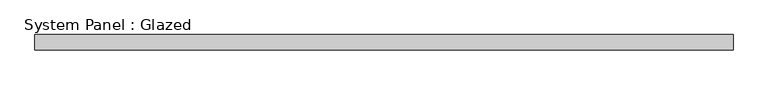
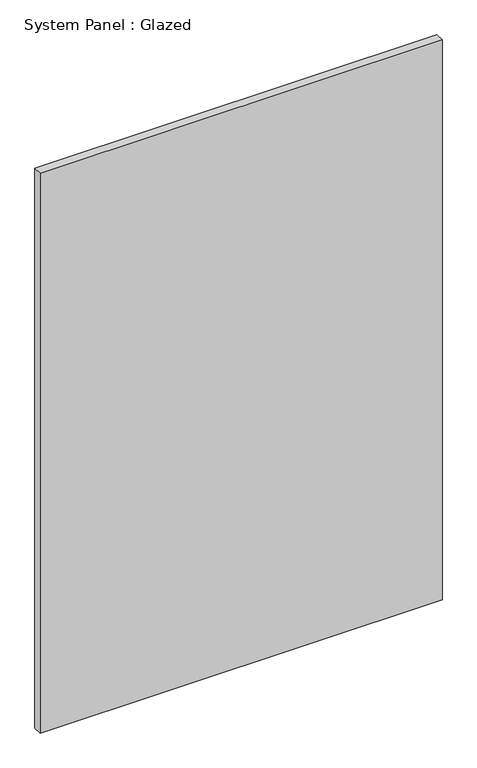
"""IFC4 building model written with IfcOpenShell, lengths in millimetres: plate geometry, System Panel : Glazed."""

from ifc_helpers import new_model, si_unit, origin, origin_with_axes, place, context, project, spatial, polyline, outline, extrude, source, transform, mapped, element, save


def system_panel_glazed_6bf442e5(model_context):
    return source(origin(), model_context, "Body", "SweptSolid", [
        extrude(outline(polyline([(577.85, 19.05), (-577.85, 19.05), (-577.85, 44.45), (577.85, 44.45), (577.85, 19.05)])), origin_with_axes(), (0.0, 0.0, 1.0), 1701.8),
    ])


if __name__ == "__main__":
    model = new_model("IFC4")
    model_context = context("Model", 3, world=origin())
    ifc_project = project(units=[si_unit("LENGTHUNIT", "METRE", prefix="MILLI")], contexts=[model_context])
    site = spatial("IfcSite", under=ifc_project)
    building = spatial("IfcBuilding", under=site)
    placement = place(None, origin())
    system_panel_glazed_shape = system_panel_glazed_6bf442e5(model_context)
    element("IfcPlate", 1, ObjectType="System Panel : Glazed", at=placement, inside=building, context=model_context, shape_type="MappedRepresentation", body=[
        mapped(system_panel_glazed_shape, transform((0.0, 0.0, 0.0), x_axis=(1.0, 0.0, 0.0), y_axis=(0.0, 1.0, 0.0), z_axis=(0.0, 0.0, 1.0))),
    ])
    save(model, "model.ifc")

# Revit data of these elements
# Type "System Panel : Glazed"
#   Construction Type Id = "GSP4R"
#   Analytic Construction = "1/8 in Pilkington single glazing"
#   Visual Light Transmittance = 0.9
#   Solar Heat Gain Coefficient = 0.86
#   Heat Transfer Coefficient (U) = 1.18115 BTU/(h·ft²·°F)
#   Define Thermal Properties by = 1
# Element 1 (IfcPlate, "System Panel : Glazed")
#   Materials on its faces: "Glass"
# Materials
#   "Glass": class "Glass", colour RGB 0 128 192, transparency 0.75, Description = "Soda Lime Glass", Cost = 0
